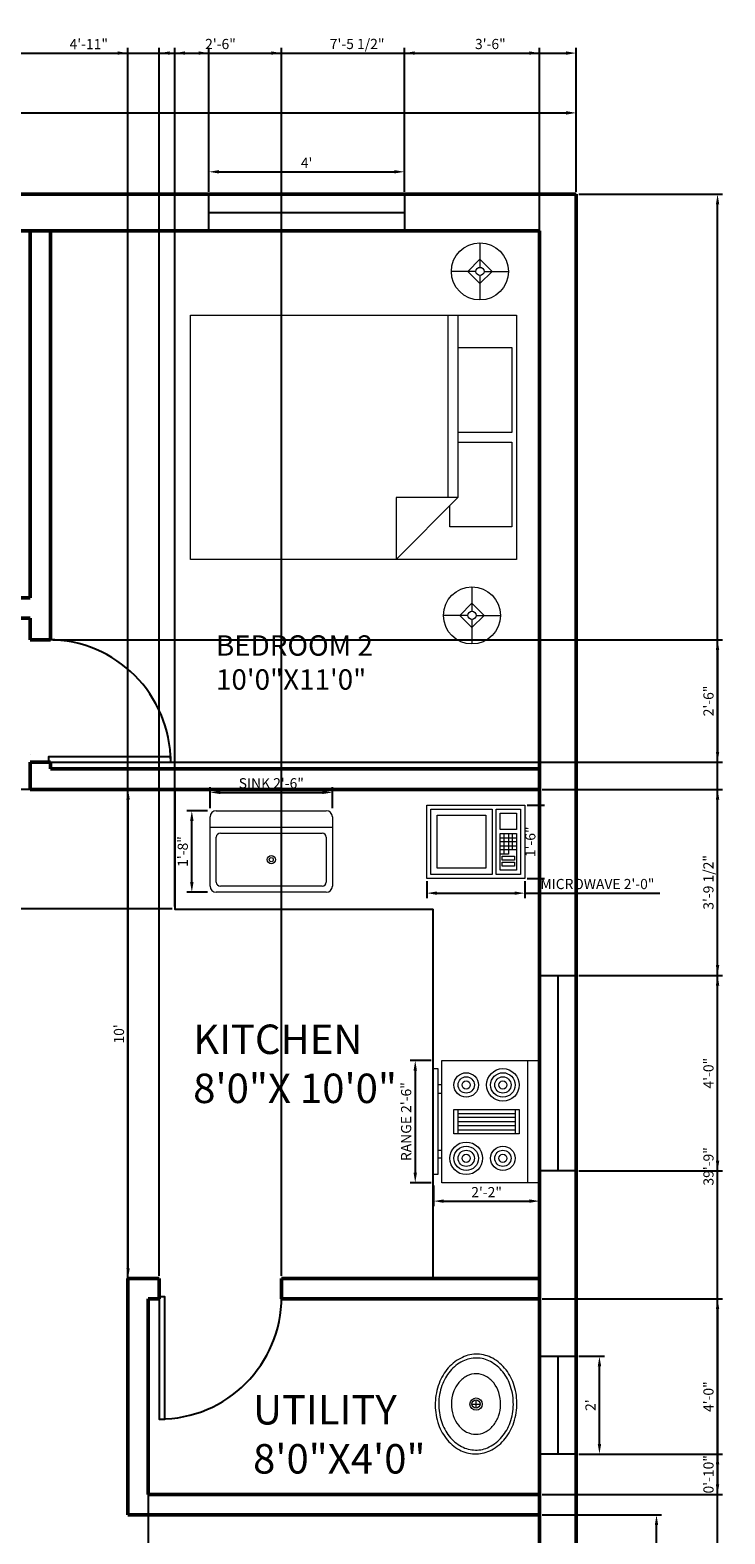
# Model space of a CAD drawing. Units: inches. Extents: x 25547 to 25983, y 30413 to 31159.
# Tile 5 of 5: x 25813 to 25983, y 30790 to 31159. Entities that reach past the tile are written whole.
import ezdxf

# ---------------------------------------------------------------- set-up
doc = ezdxf.new("R2010")
doc.units = ezdxf.units.IN
for name, color, linetype, lineweight in [('A-AREA-IDEN', 11, 'Continuous', 25), ('A-EQPM', 6, 'Continuous', 18), ('A-FLOR-CASE', 8, 'Continuous', 25), ('A-FLOR-FIXT', 6, 'Continuous', 18), ('A-WALL', 7, 'Continuous', 50), ('DIM', 4, 'Continuous', 18), ('DOOR', 3, 'Continuous', 25), ('FURNITURES', 6, 'Continuous', 18), ('WINDOW', 1, 'Continuous', 25)]:
    doc.layers.add(name, color=color, linetype=linetype, lineweight=lineweight)
doc.styles.get("Standard").update_dxf_attribs({"font": 'arial.ttf'})
doc.dimstyles.new('ISO-25', dxfattribs={"dimtxt": 2.5, "dimasz": 2.5, "dimexe": 1.25, "dimexo": 0.625, "dimtad": 1, "dimlunit": 3, "dimtxsty": 'Standard', "dimcen": 2.5, "dimadec": 0, "dimazin": 0, "dimtfac": 1, "dimtmove": 0, "dimatfit": 3, "dimfxl": 1, "dimarcsym": 0})

# ---------------------------------------------------------------- blocks, each defined once
blk = doc.blocks.new('*U4')
for p, q in [((0, 0), (0, 6)), ((40, 0), (40, 6))]:
    blk.add_line(p, q)
blk.add_lwpolyline([(0, 0), (0, -40), (1.75, -40), (1.75, 0)], close=True)
blk.add_arc((0, 0), 40, 270, 360)
blk = doc.blocks.new('Range-Oven - 30 in top')
for p, q in [((0, -3), (30, -3)), ((12, -6), (18, -6)), ((13, -20), (13, -6)), ((14, -6), (14, -20)), ((15, -20), (15, -6)), ((16, -6), (16, -20)), ((17, -20), (17, -6)), ((18, -20), (12, -20)), ((6, -24), (6, -25)), ((8, -25), (8, -24)), ((22, -25), (22, -24)), ((24, -24), (24, -25))]:
    blk.add_line(p, q)
for points in [[(0, -24), (0, 0), (30, 0), (30, -24)], [(12, -21), (12, -5), (18, -5), (18, -21)], [(2, -26), (2, -25), (28, -25), (28, -26)]]:
    blk.add_lwpolyline(points, close=True)
for centre, radius in [((6, -9), 4), ((6, -9), 3), ((6, -9), 2), ((24, -9), 3), ((24, -9), 2), ((6, -9), 1), ((24, -9), 1), ((24, -18), 4), ((6, -18), 3), ((6, -18), 2), ((6, -18), 1), ((24, -18), 3), ((24, -18), 2), ((24, -18), 1)]:
    blk.add_circle(centre, radius)
blk = doc.blocks.new('Microwave')
for p, q in [((18, 10), (22, 10)), ((22, 9), (18, 9)), ((18, 8), (22, 8)), ((19, 7), (19, 11)), ((20, 11), (20, 7)), ((21, 7), (21, 11)), ((22, 7), (18, 7)), ((20, 6), (18, 6)), ((19, 6), (19, 7)), ((20, 7), (20, 6))]:
    blk.add_line(p, q)
for points in [[(0, 0), (0, 18), (24, 18), (24, 0)], [(1, 1), (1, 17), (16, 17), (16, 1)], [(2.5, 2.5), (2.5, 15.5), (14.5, 15.5), (14.5, 2.5)], [(17, 1), (17, 17), (23, 17), (23, 1)], [(18, 12), (18, 16), (22, 16), (22, 12)], [(18, 2), (18, 11), (22, 11), (22, 2)], [(18.5, 4.5), (18.5, 5.5), (21.5, 5.5), (21.5, 4.5)], [(18.5, 3), (18.5, 4), (21.5, 4), (21.5, 3)]]:
    blk.add_lwpolyline(points, close=True)
blk = doc.blocks.new('Sink-single - 30 in top')
blk.add_line((-15, -3.999996), (15, -3.999996))
for points in [[(-13.5, 0), (13.5, 0)], [(-15, -18.499996), (-15, -1.5)], [(15, -1.5), (15, -18.499996)], [(-13.5, -17.499996), (-13.5, -6.499996)], [(-12.5, -5.499996), (12.5, -5.499996)], [(13.5, -6.499996), (13.5, -17.499996)], [(13.5, -19.999996), (-13.5, -19.999996)], [(12.5, -18.499996), (-12.5, -18.499996)]]:
    blk.add_lwpolyline(points)
for radius in [1, 0.5]:
    blk.add_circle((0, -11.999996), radius)
for centre, radius, start, end in [((-13.5, -1.5), 1.5, 90, 180), ((13.5, -1.5), 1.5, 0, 90), ((-12.5, -6.499996), 1, 90, 180), ((12.5, -6.499996), 1, 0, 90), ((-12.5, -17.499996), 1, 180, 270), ((12.5, -17.499996), 1, 270, 0), ((-13.5, -18.499996), 1.5, 180, 270), ((13.5, -18.499996), 1.5, 270, 0)]:
    blk.add_arc(centre, radius, start, end)
blk = doc.blocks.new('Bed - Queen')
for p, q in [((0, -80.00003), (0, 0)), ((0, 0), (59.99999, 0)), ((59.99999, 0), (59.99999, -80.00003)), ((7.99999, -1.2), (28.79998, -1.2)), ((7.99999, -14.4), (7.99999, -1.2)), ((28.79998, -1.2), (28.79998, -14.4)), ((31.19999, -1.2), (51.99999, -1.2)), ((31.19999, -14.4), (31.19999, -1.2)), ((51.99999, -1.2), (51.99999, -16.4)), ((0, -14.4), (44.8, -14.4)), ((59.99999, -29.6), (44.8, -14.4)), ((44.8, -14.4), (44.8, -29.6)), ((44.8, -16.8), (0, -16.8)), ((51.99999, -16.4), (46.79936, -16.4)), ((44.8, -29.6), (59.99999, -29.6)), ((59.99999, -80.00003), (0, -80.00003))]:
    blk.add_line(p, q)
blk = doc.blocks.new('Lamp - Table')
for p, q in [((0, 7), (0, 1)), ((-1, 0), (-7, 0)), ((0, 3), (-3, 0)), ((-3, 0), (0, -3)), ((3, 0), (0, 3)), ((0, -3), (3, 0)), ((1, 0), (7, 0)), ((0, -1), (0, -7))]:
    blk.add_line(p, q)
for radius in [7, 1]:
    blk.add_circle((0, 0), radius)
blk = doc.blocks.new('Sink - Oval top')
for p, q in [((-1, 0), (1, 0)), ((0, 1), (0, -1))]:
    blk.add_line(p, q)
for points in [[(-12.23, 0.39, 0.117634), (-11.46, -3.36, 0.104469), (-8.88, -6.8, 0.090016), (-5.08, -9.07, 0.08192), (-0.32, -10.02, 0.08192), (4.49, -9.38, 0.090016), (8.42, -7.36, 0.104469), (11.22, -4.09, 0.117634), (12.23, -0.39, 0.117634), (11.46, 3.36, 0.104469), (8.88, 6.8, 0.090016), (5.08, 9.07, 0.08192), (0.32, 10.02, 0.08192), (-4.49, 9.38, 0.090016), (-8.42, 7.36, 0.104469), (-11.22, 4.09, 0.117634)], [(-11.29, 0.16, 0.118622), (-10.52, -3.25, 0.104678), (-8.07, -6.36, 0.089562), (-4.54, -8.37, 0.081185), (-0.13, -9.15, 0.081185), (4.3, -8.49, 0.089562), (7.89, -6.58, 0.104678), (10.42, -3.55, 0.118622), (11.29, -0.16, 0.118622), (10.52, 3.25, 0.104678), (8.07, 6.36, 0.089562), (4.54, 8.37, 0.081185), (0.13, 9.15, 0.081185), (-4.3, 8.49, 0.089562), (-7.89, 6.58, 0.104678), (-10.42, 3.55, 0.118622)], [(-7.42, 0.08, 0.118283), (-6.91, -2.17, 0.104607), (-5.29, -4.21, 0.089718), (-2.97, -5.53, 0.081436), (-0.07, -6.04, 0.081436), (2.84, -5.59, 0.089718), (5.2, -4.33, 0.104607), (6.86, -2.32, 0.118283), (7.42, -0.08, 0.118283), (6.91, 2.17, 0.104607), (5.29, 4.21, 0.089718), (2.97, 5.53, 0.081436), (0.07, 6.04, 0.081436), (-2.84, 5.59, 0.089718), (-5.2, 4.33, 0.104607), (-6.86, 2.32, 0.118283)]]:
    blk.add_lwpolyline(points, format="xyb", close=True)
for radius in [1.5, 1]:
    blk.add_circle((0, 0), radius)
blk = doc.blocks.new('*D23')
at = {"layer": 'Defpoints', "color": 0, "transparency": 16777216}
for p in [(25946.53, 31138.79), (25587.53, 31118.83), (25946.53, 31118.83)]:
    blk.add_point(p, dxfattribs=at)
at = {"layer": 'DIM', "color": 0, "lineweight": -2, "transparency": 16777216}
for p, q in [((25587.53, 31119.45), (25587.53, 31140.04)), ((25946.53, 31119.45), (25946.53, 31140.04)), ((25590.03, 31138.79), (25944.03, 31138.79))]:
    blk.add_line(p, q, dxfattribs=at)
at = {"layer": 'DIM', "color": 0, "transparency": 16777216}
for points in [[(25590.03, 31139.21), (25590.03, 31138.37), (25587.53, 31138.79)], [(25944.03, 31139.21), (25944.03, 31138.37), (25946.53, 31138.79)]]:
    blk.add_solid(points, dxfattribs=at)
at = {"layer": 'DIM', "color": 0, "transparency": 16777216, "insert": (25767.03, 31140.69), "char_height": 2.5, "attachment_point": 5}
blk.add_mtext('29\'-11"', dxfattribs=at)
blk = doc.blocks.new('*D28')
at = {"layer": 'Defpoints', "color": 0, "transparency": 16777216}
for p in [(25937.53, 30794.83), (25966.22, 30794.83), (25937.53, 30650.83)]:
    blk.add_point(p, dxfattribs=at)
at = {"layer": 'DIM', "color": 0, "lineweight": -2, "transparency": 16777216}
for p, q in [((25938.15, 30794.83), (25967.47, 30794.83)), ((25966.22, 30653.33), (25966.22, 30792.33)), ((25938.15, 30650.83), (25967.47, 30650.83))]:
    blk.add_line(p, q, dxfattribs=at)
at = {"layer": 'DIM', "color": 0, "transparency": 16777216}
for points in [[(25965.8, 30792.33), (25966.63, 30792.33), (25966.22, 30794.83)], [(25965.8, 30653.33), (25966.63, 30653.33), (25966.22, 30650.83)]]:
    blk.add_solid(points, dxfattribs=at)
at = {"layer": 'DIM', "color": 0, "transparency": 16777216, "insert": (25964.34, 30722.83), "char_height": 2.5, "attachment_point": 5, "rotation": 90}
blk.add_mtext("12'", dxfattribs=at)
blk = doc.blocks.new('*D29')
at = {"layer": 'Defpoints', "color": 0, "transparency": 16777216}
for p in [(25946.53, 30833.75), (25952.22, 30833.75), (25946.53, 30809.75)]:
    blk.add_point(p, dxfattribs=at)
at = {"layer": 'DIM', "color": 0, "lineweight": -2, "transparency": 16777216}
for p, q in [((25947.15, 30833.75), (25953.47, 30833.75)), ((25952.22, 30812.25), (25952.22, 30831.25)), ((25947.15, 30809.75), (25953.47, 30809.75))]:
    blk.add_line(p, q, dxfattribs=at)
at = {"layer": 'DIM', "color": 0, "transparency": 16777216}
for points in [[(25951.81, 30831.25), (25952.64, 30831.25), (25952.22, 30833.75)], [(25951.81, 30812.25), (25952.64, 30812.25), (25952.22, 30809.75)]]:
    blk.add_solid(points, dxfattribs=at)
at = {"layer": 'DIM', "color": 0, "transparency": 16777216, "insert": (25950.34, 30821.76), "char_height": 2.5, "attachment_point": 5, "rotation": 90}
blk.add_mtext("2'", dxfattribs=at)
blk = doc.blocks.new('*D30')
at = {"layer": 'Defpoints', "color": 0, "transparency": 16777216}
for p in [(25836.53, 30972.83), (25836.57, 30972.83), (25836.53, 30852.83)]:
    blk.add_point(p, dxfattribs=at)
at = {"layer": 'DIM', "color": 0, "lineweight": -2, "transparency": 16777216}
for p, q in [((25836.57, 30855.33), (25836.57, 30970.33)), ((25837.15, 30972.83), (25837.82, 30972.83)), ((25837.15, 30852.83), (25837.82, 30852.83))]:
    blk.add_line(p, q, dxfattribs=at)
at = {"layer": 'DIM', "color": 0, "transparency": 16777216}
for points in [[(25836.15, 30970.33), (25836.98, 30970.33), (25836.57, 30972.83)], [(25836.15, 30855.33), (25836.98, 30855.33), (25836.57, 30852.83)]]:
    blk.add_solid(points, dxfattribs=at)
at = {"layer": 'DIM', "color": 0, "transparency": 16777216, "insert": (25834.66, 30912.83), "char_height": 2.5, "attachment_point": 5, "rotation": 90}
blk.add_mtext("10'", dxfattribs=at)
blk = doc.blocks.new('*D33')
at = {"layer": 'Defpoints', "color": 0, "transparency": 16777216}
for p in [(25904.38, 31124.34), (25856.38, 31118.83), (25904.38, 31118.83)]:
    blk.add_point(p, dxfattribs=at)
at = {"layer": 'DIM', "color": 0, "lineweight": -2, "transparency": 16777216}
for p, q in [((25856.38, 31119.45), (25856.38, 31125.59)), ((25904.38, 31119.45), (25904.38, 31125.59)), ((25858.88, 31124.34), (25901.88, 31124.34))]:
    blk.add_line(p, q, dxfattribs=at)
at = {"layer": 'DIM', "color": 0, "transparency": 16777216}
for points in [[(25858.88, 31124.76), (25858.88, 31123.93), (25856.38, 31124.34)], [(25901.88, 31124.76), (25901.88, 31123.93), (25904.38, 31124.34)]]:
    blk.add_solid(points, dxfattribs=at)
at = {"layer": 'DIM', "color": 0, "transparency": 16777216, "insert": (25880.38, 31126.22), "char_height": 2.5, "attachment_point": 5}
blk.add_mtext("4'", dxfattribs=at)
blk = doc.blocks.new('WIN-48IN')
blk.add_line((4.5, 48), (4.5, 0))
blk.add_lwpolyline([(0, 48), (9, 48), (9, 0), (0, 0)], close=True)
blk = doc.blocks.new('WIN-24IN')
blk.add_line((0, 4.5), (24, 4.5))
blk.add_lwpolyline([(0, 0), (0, 9), (24, 9), (24, 0)], close=True)
blk = doc.blocks.new('*D52')
at = {"layer": 'Defpoints', "color": 0, "transparency": 16777216}
for p in [(25911.53, 30906.31), (25907.03, 30876.31), (25911.53, 30876.31)]:
    blk.add_point(p, dxfattribs=at)
at = {"layer": 'DIM', "color": 0, "lineweight": -2, "transparency": 16777216}
for p, q in [((25910.9, 30906.31), (25905.78, 30906.31)), ((25907.03, 30903.81), (25907.03, 30878.81)), ((25910.9, 30876.31), (25905.78, 30876.31))]:
    blk.add_line(p, q, dxfattribs=at)
at = {"layer": 'DIM', "color": 0, "transparency": 16777216}
for points in [[(25906.61, 30903.81), (25907.44, 30903.81), (25907.03, 30906.31)], [(25906.61, 30878.81), (25907.44, 30878.81), (25907.03, 30876.31)]]:
    blk.add_solid(points, dxfattribs=at)
at = {"layer": 'DIM', "color": 0, "transparency": 16777216, "insert": (25905.11, 30891.31), "char_height": 2.5, "attachment_point": 5, "rotation": 90}
blk.add_mtext('RANGE 2\'-6"', dxfattribs=at)
blk = doc.blocks.new('*D53')
at = {"layer": 'Defpoints', "color": 0, "transparency": 16777216}
for p in [(25911.53, 30876.31), (25937.53, 30876.31), (25937.53, 30871.81)]:
    blk.add_point(p, dxfattribs=at)
at = {"layer": 'DIM', "color": 0, "lineweight": -2, "transparency": 16777216}
for p, q in [((25911.53, 30875.68), (25911.53, 30870.56)), ((25937.53, 30875.68), (25937.53, 30870.56)), ((25914.03, 30871.81), (25935.03, 30871.81))]:
    blk.add_line(p, q, dxfattribs=at)
at = {"layer": 'DIM', "color": 0, "transparency": 16777216}
for points in [[(25914.03, 30872.23), (25914.03, 30871.39), (25911.53, 30871.81)], [(25935.03, 30872.23), (25935.03, 30871.39), (25937.53, 30871.81)]]:
    blk.add_solid(points, dxfattribs=at)
at = {"layer": 'DIM', "color": 0, "transparency": 16777216, "insert": (25924.53, 30873.69), "char_height": 2.5, "attachment_point": 5}
blk.add_mtext('2\'-2"', dxfattribs=at)
blk = doc.blocks.new('*D54')
at = {"layer": 'Defpoints', "color": 0, "transparency": 16777216}
for p in [(25909.88, 30950.97), (25933.88, 30950.97), (25933.88, 30947.37)]:
    blk.add_point(p, dxfattribs=at)
at = {"layer": 'DIM', "color": 0, "lineweight": -2, "transparency": 16777216}
for p, q in [((25909.88, 30950.34), (25909.88, 30946.12)), ((25933.88, 30950.34), (25933.88, 30946.12)), ((25912.38, 30947.37), (25931.38, 30947.37)), ((25933.88, 30947.37), (25967.06, 30947.37))]:
    blk.add_line(p, q, dxfattribs=at)
at = {"layer": 'DIM', "color": 0, "transparency": 16777216}
for points in [[(25912.38, 30947.78), (25912.38, 30946.95), (25909.88, 30947.37)], [(25931.38, 30947.78), (25931.38, 30946.95), (25933.88, 30947.37)]]:
    blk.add_solid(points, dxfattribs=at)
at = {"layer": 'DIM', "color": 0, "transparency": 16777216, "insert": (25951.72, 30949.28), "char_height": 2.5, "attachment_point": 5}
blk.add_mtext('MICROWAVE 2\'-0"', dxfattribs=at)
blk = doc.blocks.new('*D55')
at = {"layer": 'Defpoints', "color": 0, "transparency": 16777216}
for p in [(25933.88, 30968.97), (25937.48, 30968.97), (25933.88, 30950.97)]:
    blk.add_point(p, dxfattribs=at)
at = {"layer": 'DIM', "color": 0, "lineweight": -2, "transparency": 16777216}
for p, q in [((25934.51, 30968.97), (25938.73, 30968.97)), ((25937.48, 30953.47), (25937.48, 30966.47)), ((25934.51, 30950.97), (25938.73, 30950.97))]:
    blk.add_line(p, q, dxfattribs=at)
at = {"layer": 'DIM', "color": 0, "transparency": 16777216}
for points in [[(25937.07, 30966.47), (25937.9, 30966.47), (25937.48, 30968.97)], [(25937.07, 30953.47), (25937.9, 30953.47), (25937.48, 30950.97)]]:
    blk.add_solid(points, dxfattribs=at)
at = {"layer": 'DIM', "color": 0, "transparency": 16777216, "insert": (25935.58, 30959.97), "char_height": 2.5, "attachment_point": 5, "rotation": 90}
blk.add_mtext('1\'-6"', dxfattribs=at)
blk = doc.blocks.new('*D56')
at = {"layer": 'Defpoints', "color": 0, "transparency": 16777216}
for p in [(25886.71, 30972.08), (25856.71, 30967.58), (25886.71, 30967.58)]:
    blk.add_point(p, dxfattribs=at)
at = {"layer": 'DIM', "color": 0, "lineweight": -2, "transparency": 16777216}
for p, q in [((25856.71, 30968.21), (25856.71, 30973.33)), ((25859.21, 30972.08), (25884.21, 30972.08)), ((25886.71, 30968.21), (25886.71, 30973.33))]:
    blk.add_line(p, q, dxfattribs=at)
at = {"layer": 'DIM', "color": 0, "transparency": 16777216}
for points in [[(25859.21, 30972.5), (25859.21, 30971.67), (25856.71, 30972.08)], [(25884.21, 30972.5), (25884.21, 30971.67), (25886.71, 30972.08)]]:
    blk.add_solid(points, dxfattribs=at)
at = {"layer": 'DIM', "color": 0, "transparency": 16777216, "insert": (25871.71, 30974), "char_height": 2.5, "attachment_point": 5}
blk.add_mtext('SINK 2\'-6"', dxfattribs=at)
blk = doc.blocks.new('*D57')
at = {"layer": 'Defpoints', "color": 0, "transparency": 16777216}
for p in [(25852.21, 30967.58), (25856.71, 30967.58), (25856.71, 30947.58)]:
    blk.add_point(p, dxfattribs=at)
at = {"layer": 'DIM', "color": 0, "lineweight": -2, "transparency": 16777216}
for p, q in [((25856.08, 30967.58), (25850.96, 30967.58)), ((25852.21, 30950.08), (25852.21, 30965.08)), ((25856.08, 30947.58), (25850.96, 30947.58))]:
    blk.add_line(p, q, dxfattribs=at)
at = {"layer": 'DIM', "color": 0, "transparency": 16777216}
for points in [[(25851.79, 30965.08), (25852.63, 30965.08), (25852.21, 30967.58)], [(25851.79, 30950.08), (25852.63, 30950.08), (25852.21, 30947.58)]]:
    blk.add_solid(points, dxfattribs=at)
at = {"layer": 'DIM', "color": 0, "transparency": 16777216, "insert": (25850.31, 30957.58), "char_height": 2.5, "attachment_point": 5, "rotation": 90}
blk.add_mtext('1\'-8"', dxfattribs=at)
blk = doc.blocks.new('*D70')
at = {"layer": 'Defpoints', "color": 0, "transparency": 16777216}
for p in [(25946.53, 31118.83), (25981.19, 31118.83), (25946.53, 30641.83)]:
    blk.add_point(p, dxfattribs=at)
at = {"layer": 'DIM', "color": 0, "lineweight": -2, "transparency": 16777216}
for p, q in [((25947.15, 31118.83), (25982.44, 31118.83)), ((25981.19, 30644.33), (25981.19, 31116.33)), ((25947.15, 30641.83), (25982.44, 30641.83))]:
    blk.add_line(p, q, dxfattribs=at)
at = {"layer": 'DIM', "color": 0, "transparency": 16777216}
for points in [[(25980.78, 31116.33), (25981.61, 31116.33), (25981.19, 31118.83)], [(25980.78, 30644.33), (25981.61, 30644.33), (25981.19, 30641.83)]]:
    blk.add_solid(points, dxfattribs=at)
at = {"layer": 'DIM', "color": 0, "transparency": 16777216, "insert": (25979.29, 30880.33), "char_height": 2.5, "attachment_point": 5, "rotation": 90}
blk.add_mtext('39\'-9"', dxfattribs=at)
blk = doc.blocks.new('*D75')
at = {"layer": 'Defpoints', "color": 0, "transparency": 16777216}
for p in [(25856.38, 31153.47), (25797.49, 31118.83), (25856.38, 31118.83)]:
    blk.add_point(p, dxfattribs=at)
at = {"layer": 'DIM', "color": 0, "lineweight": -2, "transparency": 16777216}
for p, q in [((25797.49, 31119.45), (25797.49, 31154.72)), ((25856.38, 31119.45), (25856.38, 31154.72)), ((25799.99, 31153.47), (25853.88, 31153.47))]:
    blk.add_line(p, q, dxfattribs=at)
at = {"layer": 'DIM', "color": 0, "transparency": 16777216}
for points in [[(25799.99, 31153.88), (25799.99, 31153.05), (25797.49, 31153.47)], [(25853.88, 31153.88), (25853.88, 31153.05), (25856.38, 31153.47)]]:
    blk.add_solid(points, dxfattribs=at)
at = {"layer": 'DIM', "color": 0, "transparency": 16777216, "insert": (25826.93, 31155.35), "char_height": 2.5, "attachment_point": 5}
blk.add_mtext('4\'-11"', dxfattribs=at)
blk = doc.blocks.new('*D76')
at = {"layer": 'Defpoints', "color": 0, "transparency": 16777216}
for p in [(25946.53, 31153.47), (25904.38, 31118.83), (25946.53, 31118.83)]:
    blk.add_point(p, dxfattribs=at)
at = {"layer": 'DIM', "color": 0, "lineweight": -2, "transparency": 16777216}
for p, q in [((25904.38, 31119.45), (25904.38, 31154.72)), ((25946.53, 31119.45), (25946.53, 31154.72)), ((25906.88, 31153.47), (25944.03, 31153.47))]:
    blk.add_line(p, q, dxfattribs=at)
at = {"layer": 'DIM', "color": 0, "transparency": 16777216}
for points in [[(25906.88, 31153.88), (25906.88, 31153.05), (25904.38, 31153.47)], [(25944.03, 31153.88), (25944.03, 31153.05), (25946.53, 31153.47)]]:
    blk.add_solid(points, dxfattribs=at)
at = {"layer": 'DIM', "color": 0, "transparency": 16777216, "insert": (25925.45, 31155.37), "char_height": 2.5, "attachment_point": 5}
blk.add_mtext('3\'-6"', dxfattribs=at)
blk = doc.blocks.new('*D83')
at = {"layer": 'Defpoints', "color": 0, "transparency": 16777216}
for p in [(25841.53, 30847.83), (25937.53, 30799.83), (25937.53, 30415.19)]:
    blk.add_point(p, dxfattribs=at)
at = {"layer": 'DIM', "color": 0, "lineweight": -2, "transparency": 16777216}
for p, q in [((25841.53, 30847.2), (25841.53, 30413.94)), ((25937.53, 30799.2), (25937.53, 30413.94)), ((25844.03, 30415.19), (25935.03, 30415.19))]:
    blk.add_line(p, q, dxfattribs=at)
at = {"layer": 'DIM', "color": 0, "transparency": 16777216}
for points in [[(25844.03, 30415.61), (25844.03, 30414.77), (25841.53, 30415.19)], [(25935.03, 30415.61), (25935.03, 30414.77), (25937.53, 30415.19)]]:
    blk.add_solid(points, dxfattribs=at)
at = {"layer": 'DIM', "color": 0, "transparency": 16777216, "insert": (25889.53, 30417.09), "char_height": 2.5, "attachment_point": 5}
blk.add_mtext('8\'-0"', dxfattribs=at)
blk = doc.blocks.new('*D84')
at = {"layer": 'Defpoints', "color": 0, "transparency": 16777216}
for p in [(25937.53, 30847.83), (25937.53, 30799.83), (25981.19, 30799.83)]:
    blk.add_point(p, dxfattribs=at)
at = {"layer": 'DIM', "color": 0, "lineweight": -2, "transparency": 16777216}
for p, q in [((25938.15, 30847.83), (25982.44, 30847.83)), ((25981.19, 30845.33), (25981.19, 30802.33)), ((25938.15, 30799.83), (25982.44, 30799.83))]:
    blk.add_line(p, q, dxfattribs=at)
at = {"layer": 'DIM', "color": 0, "transparency": 16777216}
for points in [[(25980.78, 30845.33), (25981.61, 30845.33), (25981.19, 30847.83)], [(25980.78, 30802.33), (25981.61, 30802.33), (25981.19, 30799.83)]]:
    blk.add_solid(points, dxfattribs=at)
at = {"layer": 'DIM', "color": 0, "transparency": 16777216, "insert": (25979.29, 30823.83), "char_height": 2.5, "attachment_point": 5, "rotation": 90}
blk.add_mtext('4\'-0"', dxfattribs=at)
blk = doc.blocks.new('*D85')
at = {"layer": 'Defpoints', "color": 0, "transparency": 16777216}
for p in [(25937.53, 30972.83), (25981.19, 30972.83), (25946.53, 30927.2)]:
    blk.add_point(p, dxfattribs=at)
at = {"layer": 'DIM', "color": 0, "lineweight": -2, "transparency": 16777216}
for p, q in [((25938.15, 30972.83), (25982.44, 30972.83)), ((25981.19, 30929.7), (25981.19, 30970.33)), ((25947.15, 30927.2), (25982.44, 30927.2))]:
    blk.add_line(p, q, dxfattribs=at)
at = {"layer": 'DIM', "color": 0, "transparency": 16777216}
for points in [[(25980.78, 30970.33), (25981.61, 30970.33), (25981.19, 30972.83)], [(25980.78, 30929.7), (25981.61, 30929.7), (25981.19, 30927.2)]]:
    blk.add_solid(points, dxfattribs=at)
at = {"layer": 'DIM', "color": 0, "transparency": 16777216, "insert": (25979.28, 30950.01), "char_height": 2.5, "attachment_point": 5, "rotation": 90}
blk.add_mtext('3\'-9 1/2"', dxfattribs=at)
blk = doc.blocks.new('*D90')
at = {"layer": 'Defpoints', "color": 0, "transparency": 16777216}
for p in [(25874.24, 31153.47), (25844.24, 30852.83), (25874.24, 30852.83)]:
    blk.add_point(p, dxfattribs=at)
at = {"layer": 'DIM', "color": 0, "lineweight": -2, "transparency": 16777216}
for p, q in [((25844.24, 30853.45), (25844.24, 31154.72)), ((25874.24, 30853.45), (25874.24, 31154.72)), ((25846.74, 31153.47), (25871.74, 31153.47))]:
    blk.add_line(p, q, dxfattribs=at)
at = {"layer": 'DIM', "color": 0, "transparency": 16777216}
for points in [[(25846.74, 31153.88), (25846.74, 31153.05), (25844.24, 31153.47)], [(25871.74, 31153.88), (25871.74, 31153.05), (25874.24, 31153.47)]]:
    blk.add_solid(points, dxfattribs=at)
at = {"layer": 'DIM', "color": 0, "transparency": 16777216, "insert": (25859.24, 31155.37), "char_height": 2.5, "attachment_point": 5}
blk.add_mtext('2\'-6"', dxfattribs=at)
blk = doc.blocks.new('*D91')
at = {"layer": 'Defpoints', "color": 0, "transparency": 16777216}
for p in [(25937.53, 31153.47), (25937.53, 30972.83), (25848.01, 30943.48)]:
    blk.add_point(p, dxfattribs=at)
at = {"layer": 'DIM', "color": 0, "lineweight": -2, "transparency": 16777216}
for p, q in [((25848.01, 30944.1), (25848.01, 31154.72)), ((25937.53, 30973.45), (25937.53, 31154.72)), ((25850.51, 31153.47), (25935.03, 31153.47))]:
    blk.add_line(p, q, dxfattribs=at)
at = {"layer": 'DIM', "color": 0, "transparency": 16777216}
for points in [[(25850.51, 31153.88), (25850.51, 31153.05), (25848.01, 31153.47)], [(25935.03, 31153.88), (25935.03, 31153.05), (25937.53, 31153.47)]]:
    blk.add_solid(points, dxfattribs=at)
at = {"layer": 'DIM', "color": 0, "transparency": 16777216, "insert": (25892.77, 31155.38), "char_height": 2.5, "attachment_point": 5}
blk.add_mtext('7\'-5 1/2"', dxfattribs=at)
blk = doc.blocks.new('*D92')
at = {"layer": 'Defpoints', "color": 0, "transparency": 16777216}
for p in [(25848.01, 30972.83), (25552.89, 30943.48), (25848.01, 30943.48)]:
    blk.add_point(p, dxfattribs=at)
at = {"layer": 'DIM', "color": 0, "lineweight": -2, "transparency": 16777216}
for p, q in [((25847.38, 30972.83), (25551.64, 30972.83)), ((25552.89, 30970.33), (25552.89, 30945.98)), ((25847.38, 30943.48), (25551.64, 30943.48))]:
    blk.add_line(p, q, dxfattribs=at)
at = {"layer": 'DIM', "color": 0, "transparency": 16777216}
for points in [[(25552.47, 30970.33), (25553.31, 30970.33), (25552.89, 30972.83)], [(25552.47, 30945.98), (25553.31, 30945.98), (25552.89, 30943.48)]]:
    blk.add_solid(points, dxfattribs=at)
at = {"layer": 'DIM', "color": 0, "transparency": 16777216, "insert": (25550.97, 30958.15), "char_height": 2.5, "attachment_point": 5, "rotation": 90}
blk.add_mtext('2\'-5 1/2"', dxfattribs=at)
blk = doc.blocks.new('*D93')
at = {"layer": 'Defpoints', "color": 0, "transparency": 16777216}
for p in [(25946.53, 30927.2), (25981.19, 30927.2), (25946.53, 30879.2)]:
    blk.add_point(p, dxfattribs=at)
at = {"layer": 'DIM', "color": 0, "lineweight": -2, "transparency": 16777216}
for p, q in [((25947.15, 30927.2), (25982.44, 30927.2)), ((25981.19, 30881.7), (25981.19, 30924.7)), ((25947.15, 30879.2), (25982.44, 30879.2))]:
    blk.add_line(p, q, dxfattribs=at)
at = {"layer": 'DIM', "color": 0, "transparency": 16777216}
for points in [[(25980.78, 30924.7), (25981.61, 30924.7), (25981.19, 30927.2)], [(25980.78, 30881.7), (25981.61, 30881.7), (25981.19, 30879.2)]]:
    blk.add_solid(points, dxfattribs=at)
at = {"layer": 'DIM', "color": 0, "transparency": 16777216, "insert": (25979.29, 30903.2), "char_height": 2.5, "attachment_point": 5, "rotation": 90}
blk.add_mtext('4\'-0"', dxfattribs=at)
blk = doc.blocks.new('*D98')
at = {"layer": 'Defpoints', "color": 0, "transparency": 16777216}
for p in [(25946.53, 30809.75), (25937.53, 30799.83), (25981.19, 30799.83)]:
    blk.add_point(p, dxfattribs=at)
at = {"layer": 'DIM', "color": 0, "lineweight": -2, "transparency": 16777216}
for p, q in [((25947.15, 30809.75), (25982.44, 30809.75)), ((25981.19, 30807.25), (25981.19, 30802.33)), ((25938.15, 30799.83), (25982.44, 30799.83))]:
    blk.add_line(p, q, dxfattribs=at)
at = {"layer": 'DIM', "color": 0, "transparency": 16777216}
for points in [[(25980.78, 30807.25), (25981.61, 30807.25), (25981.19, 30809.75)], [(25980.78, 30802.33), (25981.61, 30802.33), (25981.19, 30799.83)]]:
    blk.add_solid(points, dxfattribs=at)
at = {"layer": 'DIM', "color": 0, "transparency": 16777216, "insert": (25979.29, 30804.79), "char_height": 2.5, "attachment_point": 5, "rotation": 90}
blk.add_mtext('0\'-10"', dxfattribs=at)
blk = doc.blocks.new('*D99')
at = {"layer": 'Defpoints', "color": 0, "transparency": 16777216}
for p in [(25836.53, 31153.47), (25745.53, 30799.83), (25836.53, 30794.83)]:
    blk.add_point(p, dxfattribs=at)
at = {"layer": 'DIM', "color": 0, "lineweight": -2, "transparency": 16777216}
for p, q in [((25745.53, 30800.45), (25745.53, 31154.72)), ((25836.53, 30795.45), (25836.53, 31154.72)), ((25748.03, 31153.47), (25834.03, 31153.47))]:
    blk.add_line(p, q, dxfattribs=at)
at = {"layer": 'DIM', "color": 0, "transparency": 16777216}
for points in [[(25748.03, 31153.88), (25748.03, 31153.05), (25745.53, 31153.47)], [(25834.03, 31153.88), (25834.03, 31153.05), (25836.53, 31153.47)]]:
    blk.add_solid(points, dxfattribs=at)
at = {"layer": 'DIM', "color": 0, "transparency": 16777216, "insert": (25791.03, 31155.34), "char_height": 2.5, "attachment_point": 5}
blk.add_mtext('7\'-7"', dxfattribs=at)
blk = doc.blocks.new('*D101')
at = {"layer": 'Defpoints', "color": 0, "transparency": 16777216}
for p in [(25817.53, 31009.52), (25817.53, 30979.52), (25981.19, 30979.52)]:
    blk.add_point(p, dxfattribs=at)
at = {"layer": 'DIM', "color": 0, "lineweight": -2, "transparency": 16777216}
for p, q in [((25818.15, 31009.52), (25982.44, 31009.52)), ((25981.19, 31007.02), (25981.19, 30982.02)), ((25818.15, 30979.52), (25982.44, 30979.52))]:
    blk.add_line(p, q, dxfattribs=at)
at = {"layer": 'DIM', "color": 0, "transparency": 16777216}
for points in [[(25980.78, 31007.02), (25981.61, 31007.02), (25981.19, 31009.52)], [(25980.78, 30982.02), (25981.61, 30982.02), (25981.19, 30979.52)]]:
    blk.add_solid(points, dxfattribs=at)
at = {"layer": 'DIM', "color": 0, "transparency": 16777216, "insert": (25979.29, 30994.52), "char_height": 2.5, "attachment_point": 5, "rotation": 90}
blk.add_mtext('2\'-6"', dxfattribs=at)

msp = doc.modelspace()

# ---------------------------------------------------------------- linework, layer by layer
at = {"layer": 'A-FLOR-CASE'}
for points in [[(25937.528, 30943.478), (25937.528, 30972.828), (25848.008, 30972.828), (25848.008, 30943.478), (25911.431, 30943.478)], [(25911.431, 30972.828), (25937.528, 30972.828), (25937.528, 30852.828), (25911.431, 30852.828), (25911.431, 30943.478)]]:
    msp.add_lwpolyline(points, dxfattribs=at)
at = {"layer": 'A-WALL'}
for p, q in [((25587.528, 31118.828), (25946.528, 31118.828)), ((25946.528, 30585.868), (25946.528, 31118.828)), ((25596.528, 31109.828), (25937.528, 31109.828)), ((25812.528, 31019.828), (25812.528, 31109.828)), ((25817.528, 31009.519), (25817.528, 31109.828)), ((25937.528, 30594.868), (25937.528, 31109.828)), ((25808.126, 31019.828), (25812.528, 31019.828)), ((25808.126, 31014.828), (25812.528, 31014.828)), ((25812.528, 31009.519), (25812.528, 31014.828)), ((25812.528, 30972.828), (25812.528, 30979.519)), ((25812.528, 30979.519), (25817.528, 30979.519)), ((25817.528, 30979.523), (25817.528, 30979.519)), ((25817.528, 30977.828), (25817.528, 30979.519)), ((25817.528, 30977.828), (25937.528, 30977.828)), ((25812.528, 30972.828), (25937.528, 30972.828)), ((25836.528, 30794.828), (25836.528, 30852.828)), ((25836.528, 30852.828), (25844.239, 30852.828)), ((25836.528, 30794.828), (25836.528, 30852.828)), ((25874.239, 30852.828), (25937.528, 30852.828)), ((25841.528, 30799.828), (25841.528, 30847.828)), ((25841.528, 30847.828), (25844.239, 30847.828)), ((25841.528, 30799.828), (25841.528, 30847.828)), ((25874.239, 30847.828), (25937.528, 30847.828)), ((25841.528, 30799.828), (25937.528, 30799.828)), ((25836.528, 30794.828), (25937.528, 30794.828))]:
    msp.add_line(p, q, dxfattribs=at)
for points in [[(25812.528, 31009.519), (25812.528, 31011.496)], [(25817.528, 31011.496), (25817.528, 31009.519)], [(25812.528, 31009.519), (25817.528, 31009.519)], [(25844.239, 30847.828), (25844.239, 30852.828)], [(25874.239, 30852.828), (25874.239, 30847.828)]]:
    msp.add_lwpolyline(points, dxfattribs=at)
msp.add_lwpolyline([(25812.528, 30981.496), (25812.528, 30981.496)], close=True, dxfattribs=at)

# ---------------------------------------------------------------- block references
at = {"layer": 'A-EQPM'}
msp.add_blockref('Microwave', (25909.883, 30950.966), dxfattribs=at)
at = {"layer": 'A-EQPM', "rotation": 270}
msp.add_blockref('Range-Oven - 30 in top', (25937.528, 30906.31), dxfattribs=at)
at = {"layer": 'A-FLOR-FIXT'}
msp.add_blockref('Sink-single - 30 in top', (25871.709, 30967.582), dxfattribs=at)
at = {"layer": 'A-FLOR-FIXT', "rotation": 90}
msp.add_blockref('Sink - Oval top', (25921.944, 30822.021), dxfattribs=at)
at = {"layer": 'DOOR', "xscale": 0.75, "yscale": 0.75, "zscale": 0.75, "rotation": 90}
msp.add_blockref('*U4', (25817.028, 30979.519), dxfattribs=at)
at = {"layer": 'DOOR', "xscale": 0.75, "yscale": 0.75, "zscale": 0.75}
msp.add_blockref('*U4', (25844.239, 30848.328), dxfattribs=at)
at = {"layer": 'FURNITURES'}
for p in [(25922.897, 31099.901), (25920.943, 31015.512)]:
    msp.add_blockref('Lamp - Table', p, dxfattribs=at)
at = {"layer": 'FURNITURES', "rotation": 270}
msp.add_blockref('Bed - Queen', (25931.907, 31089.198), dxfattribs=at)
at = {"layer": 'WINDOW'}
for name, p, rotation in [('WIN-48IN', (25904.375, 31109.828), 89.99999999998533), ('WIN-24IN', (25937.528, 30833.749), 270.0000000000216)]:
    msp.add_blockref(name, p, dxfattribs=dict(at, rotation=rotation))
msp.add_blockref('WIN-48IN', (25937.528, 30879.2), dxfattribs=at)

# ---------------------------------------------------------------- texts
at = {"layer": 'A-AREA-IDEN', "attachment_point": 1}
for s, insert, char_height in [('{\\fArial|b1|i1|c0|p34;BEDROOM 2\\P10\'0"X11\'0"}', (25858.143, 31010.618), 5), ('{\\fArial|b1|i1|c0|p34;KITCHEN\\P8\'0"X 10\'0"}', (25852.547, 30915.123), 7.21917), ('{\\fArial|b1|i1|c0|p34;UTILITY\\P8\'0"X4\'0"}', (25867.23, 30824.232), 7.21917)]:
    msp.add_mtext_dynamic_manual_height_columns(s, width=113.82935, gutter_width=18.048, heights=[0], dxfattribs=dict(at, insert=insert, char_height=char_height))

# ---------------------------------------------------------------- dimensions: what is measured, and where the dimension line sits
at = {"layer": 'DIM'}
for base, p1, p2, override, picture, middle in [((25937.528, 31153.465), (25848.008, 30943.478), (25937.528, 30972.828), {"dimdec": 1, "dimlfac": 1, "dimrnd": 0, "dimzin": 1, "dimdsep": 46, "dimlunit": 4, "dimfrac": 2}, '*D91', (25892.768, 31155.383)), ((25836.528, 31153.465), (25745.528, 30799.828), (25836.528, 30794.828), {"dimdec": 1, "dimlfac": 1, "dimrnd": 0, "dimzin": 1, "dimdsep": 46, "dimlunit": 4, "dimfrac": 2}, '*D99', (25791.028, 31155.34)), ((25856.375, 31153.465), (25797.486, 31118.828), (25856.375, 31118.828), {"dimdec": 1, "dimlfac": 1, "dimrnd": 0, "dimzin": 1, "dimdsep": 46, "dimlunit": 4, "dimfrac": 2}, '*D75', (25826.931, 31155.346)), ((25874.239, 31153.465), (25844.239, 30852.828), (25874.239, 30852.828), {"dimdec": 1, "dimlfac": 1, "dimrnd": 0, "dimzin": 1, "dimdsep": 46, "dimlunit": 4, "dimfrac": 2}, '*D90', (25859.239, 31155.367)), ((25946.528, 31153.465), (25904.375, 31118.828), (25946.528, 31118.828), {"dimdec": 1, "dimlfac": 1, "dimrnd": 0, "dimzin": 1, "dimdsep": 46, "dimlunit": 4, "dimfrac": 2}, '*D76', (25925.452, 31155.368)), ((25946.528, 31138.789), (25587.528, 31118.828), (25946.528, 31118.828), {"dimclrd": 0, "dimclre": 0, "dimclrt": 0}, '*D23', (25767.028, 31140.69)), ((25904.375, 31124.344), (25856.375, 31118.828), (25904.375, 31118.828), {"dimclrd": 0, "dimclre": 0, "dimclrt": 0}, '*D33', (25880.375, 31126.219)), ((25937.528, 30871.81), (25911.528, 30876.31), (25937.528, 30876.31), {"dimdec": 1, "dimlfac": 1, "dimrnd": 0, "dimzin": 1, "dimdsep": 46, "dimlunit": 4, "dimfrac": 2}, '*D53', (25924.528, 30873.69)), ((25937.528, 30415.19), (25841.528, 30847.828), (25937.528, 30799.828), {"dimdec": 1, "dimlfac": 1, "dimrnd": 0, "dimzin": 1, "dimdsep": 46, "dimlunit": 4, "dimfrac": 2}, '*D83', (25889.528, 30417.092))]:
    dim = msp.add_linear_dim(base=base, p1=p1, p2=p2, dimstyle='ISO-25', override=override, dxfattribs=at)
    dim.commit()
    dim.dimension.update_dxf_attribs({"geometry": picture, "text_midpoint": middle})
for base, p1, p2, override, picture, middle in [((25981.195, 31118.828), (25946.528, 30641.828), (25946.528, 31118.828), {"dimdec": 1, "dimlfac": 1, "dimrnd": 0, "dimzin": 1, "dimdsep": 46, "dimlunit": 4, "dimfrac": 2}, '*D70', (25979.292, 30880.328)), ((25981.195, 30979.523), (25817.528, 31009.519), (25817.528, 30979.523), {"dimdec": 1, "dimlfac": 1, "dimrnd": 0, "dimzin": 1, "dimdsep": 46, "dimlunit": 4, "dimfrac": 2}, '*D101', (25979.293, 30994.521)), ((25552.8906, 30943.4778), (25848.0078, 30972.8279), (25848.0078, 30943.4778), {"dimdec": 1, "dimlfac": 1, "dimrnd": 0, "dimzin": 1, "dimdsep": 46, "dimlunit": 4, "dimfrac": 2}, '*D92', (25550.973, 30958.1529)), ((25836.565, 30972.828), (25836.528, 30852.828), (25836.528, 30972.828), {"dimclrd": 0, "dimclre": 0, "dimclrt": 0}, '*D30', (25834.664, 30912.828)), ((25981.195, 30972.828), (25946.528, 30927.2), (25937.528, 30972.828), {"dimdec": 1, "dimlfac": 1, "dimrnd": 0, "dimzin": 1, "dimdsep": 46, "dimlunit": 4, "dimfrac": 2}, '*D85', (25979.276, 30950.014)), ((25852.209, 30967.582), (25856.709, 30947.582), (25856.709, 30967.582), {"dimdec": 1, "dimlfac": 1, "dimrnd": 0, "dimzin": 1, "dimdsep": 46, "dimlunit": 4, "dimfrac": 2}, '*D57', (25850.307, 30957.582)), ((25937.483, 30968.966), (25933.883, 30950.966), (25933.883, 30968.966), {"dimdec": 1, "dimlfac": 1, "dimrnd": 0, "dimzin": 1, "dimdsep": 46, "dimlunit": 4, "dimfrac": 2}, '*D55', (25935.582, 30959.966)), ((25981.195, 30927.2), (25946.528, 30879.2), (25946.528, 30927.2), {"dimdec": 1, "dimlfac": 1, "dimrnd": 0, "dimzin": 1, "dimdsep": 46, "dimlunit": 4, "dimfrac": 2}, '*D93', (25979.293, 30903.2)), ((25981.195, 30799.828), (25937.528, 30847.828), (25937.528, 30799.828), {"dimdec": 1, "dimlfac": 1, "dimrnd": 0, "dimzin": 1, "dimdsep": 46, "dimlunit": 4, "dimfrac": 2}, '*D84', (25979.293, 30823.828)), ((25981.195, 30799.828), (25946.528, 30809.749), (25937.528, 30799.828), {"dimdec": 1, "dimlfac": 1, "dimrnd": 0, "dimzin": 1, "dimdsep": 46, "dimlunit": 4, "dimfrac": 2}, '*D98', (25979.293, 30804.788)), ((25966.218, 30794.828), (25937.528, 30650.828), (25937.528, 30794.828), {"dimclrd": 0, "dimclre": 0, "dimclrt": 0}, '*D28', (25964.338, 30722.828))]:
    dim = msp.add_linear_dim(base=base, p1=p1, p2=p2, angle=90, dimstyle='ISO-25', override=override, dxfattribs=at)
    dim.commit()
    dim.dimension.update_dxf_attribs({"geometry": picture, "text_midpoint": middle})
for base, p1, p2, text, picture, middle in [((25886.709, 30972.082), (25856.709, 30967.582), (25886.709, 30967.582), 'SINK <>', '*D56', (25871.709, 30974)), ((25933.883, 30947.366), (25909.883, 30950.966), (25933.883, 30950.966), 'MICROWAVE <>', '*D54', (25951.722, 30949.284))]:
    dim = msp.add_linear_dim(base=base, p1=p1, p2=p2, text=text, dimstyle='ISO-25', override={"dimdec": 1, "dimlfac": 1, "dimrnd": 0, "dimzin": 1, "dimdsep": 46, "dimlunit": 4, "dimfrac": 2}, dxfattribs=at)
    dim.commit()
    dim.dimension.update_dxf_attribs({"geometry": picture, "text_midpoint": middle})
dim = msp.add_linear_dim(base=(25907.028, 30876.31), p1=(25911.528, 30906.31), p2=(25911.528, 30876.31), angle=270, text='RANGE <>', dimstyle='ISO-25', override={"dimdec": 1, "dimlfac": 1, "dimrnd": 0, "dimzin": 1, "dimdsep": 46, "dimlunit": 4, "dimfrac": 2}, dxfattribs=at)
dim.commit()
dim.dimension.update_dxf_attribs({"geometry": '*D52', "text_midpoint": (25905.11, 30891.31)})
dim = msp.add_linear_dim(base=(25952.224, 30833.749), p1=(25946.528, 30809.749), p2=(25946.528, 30833.749), angle=90, dimstyle='ISO-25', override={"dimclrd": 0, "dimclre": 0, "dimclrt": 0}, dxfattribs=at)
dim.commit()
dim.dimension.update_dxf_attribs({"geometry": '*D29', "text_midpoint": (25952.224, 30821.758), "dimtype": 160})

doc.saveas('drawing.dxf')
